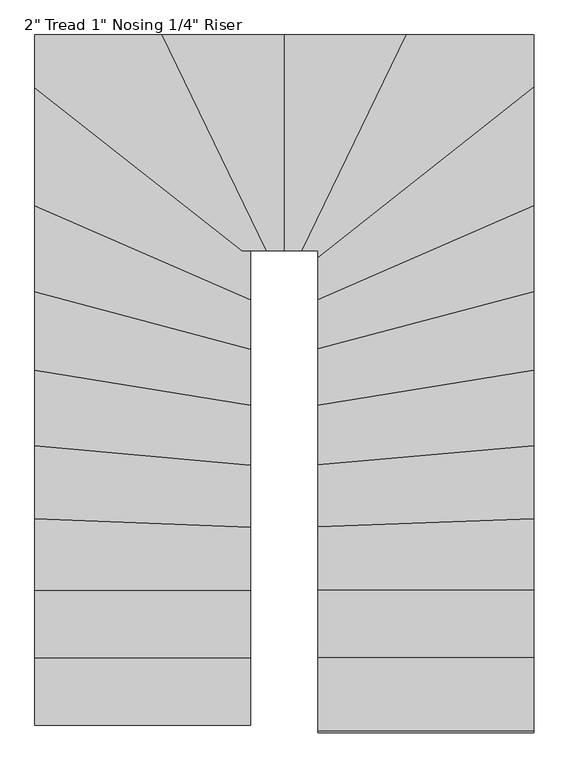
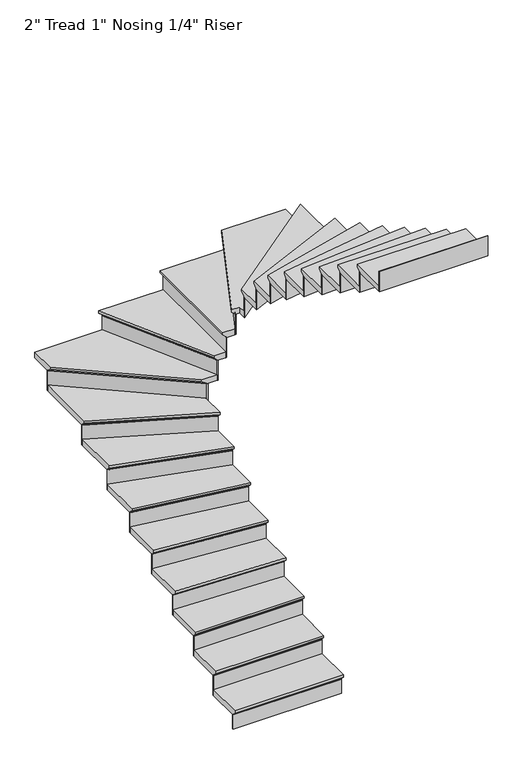
"""IFC4 building model written with IfcOpenShell, lengths in millimetres: stair flight geometry."""

from ifc_helpers import new_model, si_unit, origin, place, context, project, spatial, faceted_brep, source, transform, mapped, element, save


def stair_flight_b3d82c80(model_context):
    return source(origin(), model_context, "Body", "Brep", [
        faceted_brep([(-5047.1987704, -4554.2130548, 55019.1214286), (-5047.1987704, -4554.2130548, 55038.1714286), (-5940.8822214, -4554.2130548, 55038.1714286), (-5940.8822214, -4554.2130548, 55019.1214286), (-5047.1987704, -4528.8130548, 54993.7214286), (-5940.8822214, -4528.8130548, 54993.7214286), (-5047.1987704, -4249.4130548, 55038.1714286), (-5940.8822214, -4249.4130548, 55038.1714286), (-5940.8822214, -4528.8130548, 54987.3714286), (-5940.8822214, -4249.4130548, 54987.3714286), (-5047.1987704, -4249.4130548, 54987.3714286), (-5047.1987704, -4528.8130548, 54987.3714286)], [[[0, 1, 2, 3]], [[4, 0, 3, 5]], [[2, 1, 6, 7]], [[8, 9, 10, 11]], [[2, 7, 9, 8, 5, 3]], [[8, 11, 4, 5]], [[6, 1, 0, 4, 11, 10]], [[7, 6, 10, 9]]]),
        faceted_brep([(-5047.1987704, -4528.8130548, 54987.3714286), (-5047.1987704, -4528.8130548, 54864.0), (-5047.1987704, -4522.4630548, 54864.0), (-5047.1987704, -4522.4630548, 54987.3714286), (-5940.8822214, -4528.8130548, 54987.3714286), (-5940.8822214, -4522.4630548, 54987.3714286), (-5940.8822214, -4522.4630548, 54864.0), (-5940.8822214, -4528.8130548, 54864.0)], [[[0, 1, 2, 3]], [[4, 5, 6, 7]], [[1, 0, 4, 7]], [[2, 1, 7, 6]], [[3, 2, 6, 5]], [[0, 3, 5, 4]]]),
        faceted_brep([(-5047.1987704, -4249.4130548, 55161.5428571), (-5047.1987704, -4249.4130548, 54987.3714286), (-5047.1987704, -4243.0630548, 54987.3714286), (-5047.1987704, -4243.0630548, 55161.5428571), (-5940.8822214, -4249.4130548, 55161.5428571), (-5940.8822214, -4243.0630548, 55161.5428571), (-5940.8822214, -4243.0630548, 54987.3714286), (-5940.8822214, -4249.4130548, 54987.3714286)], [[[0, 1, 2, 3]], [[4, 5, 6, 7]], [[1, 0, 4, 7]], [[2, 1, 7, 6]], [[3, 2, 6, 5]], [[0, 3, 5, 4]]]),
        faceted_brep([(-5940.8822214, -4274.8130548, 55212.3428571), (-5047.1987704, -4274.8130548, 55212.3428571), (-5047.1987704, -3970.0130548, 55212.3428571), (-5940.8822214, -3970.0130548, 55212.3428571), (-5940.8822214, -4249.4130548, 55161.5428571), (-5940.8822214, -3970.0130548, 55161.5428571), (-5047.1987704, -3970.0130548, 55161.5428571), (-5047.1987704, -4249.4130548, 55161.5428571), (-5940.8822214, -4249.4130548, 55167.8928571), (-5940.8822214, -4274.8130548, 55193.2928571), (-5047.1987704, -4249.4130548, 55167.8928571), (-5047.1987704, -4274.8130548, 55193.2928571)], [[[0, 1, 2, 3]], [[4, 5, 6, 7]], [[0, 3, 5, 4, 8, 9]], [[4, 7, 10, 8]], [[2, 1, 11, 10, 7, 6]], [[3, 2, 6, 5]], [[11, 1, 0, 9]], [[10, 11, 9, 8]]]),
        faceted_brep([(-5047.1987704, -3970.0130548, 55335.7142857), (-5047.1987704, -3970.0130548, 55161.5428571), (-5047.1987704, -3963.6630548, 55161.5428571), (-5047.1987704, -3963.6630548, 55335.7142857), (-5940.8822214, -3970.0130548, 55335.7142857), (-5940.8822214, -3963.6630548, 55335.7142857), (-5940.8822214, -3963.6630548, 55161.5428571), (-5940.8822214, -3970.0130548, 55161.5428571)], [[[0, 1, 2, 3]], [[4, 5, 6, 7]], [[1, 0, 4, 7]], [[2, 1, 7, 6]], [[3, 2, 6, 5]], [[0, 3, 5, 4]]]),
        faceted_brep([(-5940.8822214, -3995.4130548, 55386.5142857), (-5047.1987704, -3995.4130548, 55386.5142857), (-5047.1987704, -3707.9036879, 55386.5142857), (-5940.8822214, -3673.2843203, 55386.5142857), (-5940.8822214, -3970.0130548, 55335.7142857), (-5940.8822214, -3673.2843203, 55335.7142857), (-5047.1987704, -3707.9036879, 55335.7142857), (-5047.1987704, -3970.0130548, 55335.7142857), (-5940.8822214, -3970.0130548, 55342.0642857), (-5940.8822214, -3995.4130548, 55367.4642857), (-5047.1987704, -3970.0130548, 55342.0642857), (-5047.1987704, -3995.4130548, 55367.4642857)], [[[0, 1, 2, 3]], [[4, 5, 6, 7]], [[0, 3, 5, 4, 8, 9]], [[4, 7, 10, 8]], [[2, 1, 11, 10, 7, 6]], [[3, 2, 6, 5]], [[11, 1, 0, 9]], [[10, 11, 9, 8]]]),
        faceted_brep([(-5047.1987704, -3707.9036879, 55509.8857143), (-5047.1987704, -3707.9036879, 55335.7142857), (-5047.1987704, -3701.5489252, 55335.7142857), (-5047.1987704, -3701.5489252, 55509.8857143), (-5940.8822214, -3673.2843203, 55509.8857143), (-5940.8822214, -3666.9295576, 55509.8857143), (-5940.8822214, -3666.9295576, 55335.7142857), (-5940.8822214, -3673.2843203, 55335.7142857)], [[[0, 1, 2, 3]], [[4, 5, 6, 7]], [[1, 0, 4, 7]], [[2, 1, 7, 6]], [[3, 2, 6, 5]], [[0, 3, 5, 4]]]),
        faceted_brep([(-5940.8822214, -3698.703371, 55560.6857143), (-5047.1987704, -3733.3227386, 55560.6857143), (-5047.1987704, -3451.3234819, 55560.6857143), (-5940.8822214, -3370.89733, 55560.6857143), (-5940.8822214, -3673.2843203, 55509.8857143), (-5940.8822214, -3370.89733, 55509.8857143), (-5047.1987704, -3451.3234819, 55509.8857143), (-5047.1987704, -3707.9036879, 55509.8857143), (-5940.8822214, -3673.2843203, 55516.2357143), (-5940.8822214, -3698.703371, 55541.6357143), (-5047.1987704, -3707.9036879, 55516.2357143), (-5047.1987704, -3733.3227386, 55541.6357143)], [[[0, 1, 2, 3]], [[4, 5, 6, 7]], [[0, 3, 5, 4, 8, 9]], [[4, 7, 10, 8]], [[2, 1, 11, 10, 7, 6]], [[3, 2, 6, 5]], [[11, 1, 0, 9]], [[10, 11, 9, 8]]]),
        faceted_brep([(-5047.1987704, -3451.3234819, 55684.0571429), (-5047.1987704, -3451.3234819, 55509.8857143), (-5047.1987704, -3444.9478197, 55509.8857143), (-5047.1987704, -3444.9478197, 55684.0571429), (-5940.8822214, -3370.89733, 55684.0571429), (-5940.8822214, -3364.5216678, 55684.0571429), (-5940.8822214, -3364.5216678, 55509.8857143), (-5940.8822214, -3370.89733, 55509.8857143)], [[[0, 1, 2, 3]], [[4, 5, 6, 7]], [[1, 0, 4, 7]], [[2, 1, 7, 6]], [[3, 2, 6, 5]], [[0, 3, 5, 4]]]),
        faceted_brep([(-5940.8822214, -3396.3999789, 55734.8571429), (-5047.1987704, -3476.8261308, 55734.8571429), (-5047.1987704, -3203.4301079, 55734.8571429), (-5940.8822214, -3059.5417727, 55734.8571429), (-5940.8822214, -3370.89733, 55684.0571429), (-5940.8822214, -3059.5417727, 55684.0571429), (-5047.1987704, -3203.4301079, 55684.0571429), (-5047.1987704, -3451.3234819, 55684.0571429), (-5940.8822214, -3370.89733, 55690.4071429), (-5940.8822214, -3396.3999789, 55715.8071429), (-5047.1987704, -3451.3234819, 55690.4071429), (-5047.1987704, -3476.8261308, 55715.8071429)], [[[0, 1, 2, 3]], [[4, 5, 6, 7]], [[0, 3, 5, 4, 8, 9]], [[4, 7, 10, 8]], [[2, 1, 11, 10, 7, 6]], [[3, 2, 6, 5]], [[11, 1, 0, 9]], [[10, 11, 9, 8]]]),
        faceted_brep([(-5047.1987704, -3203.4301079, 55858.2285714), (-5047.1987704, -3203.4301079, 55684.0571429), (-5047.1987704, -3196.9983292, 55684.0571429), (-5047.1987704, -3196.9983292, 55858.2285714), (-5940.8822214, -3059.5417727, 55858.2285714), (-5940.8822214, -3053.109994, 55858.2285714), (-5940.8822214, -3053.109994, 55684.0571429), (-5940.8822214, -3059.5417727, 55684.0571429)], [[[0, 1, 2, 3]], [[4, 5, 6, 7]], [[1, 0, 4, 7]], [[2, 1, 7, 6]], [[3, 2, 6, 5]], [[0, 3, 5, 4]]]),
        faceted_brep([(-5940.8822214, -3085.2688872, 55909.0285714), (-5047.1987704, -3229.1572224, 55909.0285714), (-5047.1987704, -2970.3553609, 55909.0285714), (-5940.8822214, -2732.7052783, 55909.0285714), (-5940.8822214, -3059.5417727, 55858.2285714), (-5940.8822214, -2732.7052783, 55858.2285714), (-5047.1987704, -2970.3553609, 55858.2285714), (-5047.1987704, -3203.4301079, 55858.2285714), (-5940.8822214, -3059.5417727, 55864.5785714), (-5940.8822214, -3085.2688872, 55889.9785714), (-5047.1987704, -3203.4301079, 55864.5785714), (-5047.1987704, -3229.1572224, 55889.9785714)], [[[0, 1, 2, 3]], [[4, 5, 6, 7]], [[0, 3, 5, 4, 8, 9]], [[4, 7, 10, 8]], [[2, 1, 11, 10, 7, 6]], [[3, 2, 6, 5]], [[11, 1, 0, 9]], [[10, 11, 9, 8]]]),
        faceted_brep([(-5047.1987704, -2970.3553609, 56032.4), (-5047.1987704, -2970.3553609, 55858.2285714), (-5047.1987704, -2963.7846771, 55858.2285714), (-5047.1987704, -2963.7846771, 56032.4), (-5940.8822214, -2732.7052783, 56032.4), (-5940.8822214, -2726.1345945, 56032.4), (-5940.8822214, -2726.1345945, 55858.2285714), (-5940.8822214, -2732.7052783, 55858.2285714)], [[[0, 1, 2, 3]], [[4, 5, 6, 7]], [[1, 0, 4, 7]], [[2, 1, 7, 6]], [[3, 2, 6, 5]], [[0, 3, 5, 4]]]),
        faceted_brep([(-5940.8822214, -2758.9880136, 56083.2), (-5047.1987704, -2996.6380961, 56083.2), (-5047.1987704, -2765.8050203, 56083.2), (-5940.8822214, -2375.5896532, 56083.2), (-5940.8822214, -2732.7052783, 56032.4), (-5940.8822214, -2375.5896532, 56032.4), (-5047.1987704, -2765.8050203, 56032.4), (-5047.1987704, -2970.3553609, 56032.4), (-5940.8822214, -2732.7052783, 56038.75), (-5940.8822214, -2758.9880136, 56064.15), (-5047.1987704, -2970.3553609, 56038.75), (-5047.1987704, -2996.6380961, 56064.15)], [[[0, 1, 2, 3]], [[4, 5, 6, 7]], [[0, 3, 5, 4, 8, 9]], [[4, 7, 10, 8]], [[2, 1, 11, 10, 7, 6]], [[3, 2, 6, 5]], [[11, 1, 0, 9]], [[10, 11, 9, 8]]]),
        faceted_brep([(-5047.1987704, -2765.8050203, 56206.5714286), (-5047.1987704, -2765.8050203, 56032.4), (-5047.1987704, -2758.8760908, 56032.4), (-5047.1987704, -2758.8760908, 56206.5714286), (-5940.8822214, -2375.5896532, 56206.5714286), (-5940.8822214, -2368.6607237, 56206.5714286), (-5940.8822214, -2368.6607237, 56032.4), (-5940.8822214, -2375.5896532, 56032.4)], [[[0, 1, 2, 3]], [[4, 5, 6, 7]], [[1, 0, 4, 7]], [[2, 1, 7, 6]], [[3, 2, 6, 5]], [[0, 3, 5, 4]]]),
        faceted_brep([(-5940.8822214, -2403.3053713, 56257.3714286), (-5047.1987704, -2793.5207384, 56257.3714286), (-5047.1987704, -2590.8424524, 56257.3714286), (-5040.8038639, -2590.8424524, 56257.3714286), (-5940.8822214, -1882.1944717, 56257.3714286), (-5940.8822214, -2375.5896532, 56206.5714286), (-5940.8822214, -1882.1944717, 56206.5714286), (-5040.8038639, -2590.8424524, 56206.5714286), (-5047.1987704, -2590.8424524, 56206.5714286), (-5047.1987704, -2765.8050203, 56206.5714286), (-5940.8822214, -2375.5896532, 56212.9214286), (-5940.8822214, -2403.3053713, 56238.3214286), (-5047.1987704, -2765.8050203, 56212.9214286), (-5047.1987704, -2793.5207384, 56238.3214286)], [[[0, 1, 2, 3, 4]], [[5, 6, 7, 8, 9]], [[0, 4, 6, 5, 10, 11]], [[5, 9, 12, 10]], [[2, 1, 13, 12, 9, 8]], [[4, 3, 7, 6]], [[13, 1, 0, 11]], [[12, 13, 11, 10]], [[3, 2, 8, 7]]]),
        faceted_brep([(-5040.8038639, -2590.8424524, 56380.7428571), (-5040.8038639, -2590.8424524, 56206.5714286), (-5030.5387554, -2590.8424524, 56206.5714286), (-5030.5387554, -2590.8424524, 56380.7428571), (-5940.8822214, -1882.1944717, 56380.7428571), (-5940.8822214, -1874.1125661, 56380.7428571), (-5940.8822214, -1874.1125661, 56206.5714286), (-5940.8822214, -1882.1944717, 56206.5714286)], [[[0, 1, 2, 3]], [[4, 5, 6, 7]], [[1, 0, 4, 7]], [[2, 1, 7, 6]], [[3, 2, 6, 5]], [[0, 3, 5, 4]]]),
        faceted_brep([(-5384.6489457, -1697.1590014, 56431.5428571), (-5940.8822214, -1697.1590014, 56431.5428571), (-5940.8822214, -1914.5220945, 56431.5428571), (-5081.8642978, -2590.8424524, 56431.5428571), (-4952.3566185, -2590.8424524, 56431.5428571), (-5940.8822214, -1697.1590014, 56380.7428571), (-5384.6489457, -1697.1590014, 56380.7428571), (-4952.3566185, -2590.8424524, 56380.7428571), (-5040.8038639, -2590.8424524, 56380.7428571), (-5940.8822214, -1882.1944717, 56380.7428571), (-5940.8822214, -1882.1944717, 56387.0928571), (-5940.8822214, -1914.5220945, 56412.4928571), (-5040.8038639, -2590.8424524, 56387.0928571), (-5081.8642978, -2590.8424524, 56412.4928571)], [[[0, 1, 2, 3, 4]], [[5, 6, 7, 8, 9]], [[1, 0, 6, 5]], [[2, 1, 5, 9, 10, 11]], [[9, 8, 12, 10]], [[4, 3, 13, 12, 8, 7]], [[0, 4, 7, 6]], [[13, 3, 2, 11]], [[12, 13, 11, 10]]]),
        faceted_brep([(-4952.3566185, -2590.8424524, 56554.9142857), (-4952.3566185, -2590.8424524, 56380.7428571), (-4945.3027294, -2590.8424524, 56380.7428571), (-4945.3027294, -2590.8424524, 56554.9142857), (-5384.6489457, -1697.1590014, 56554.9142857), (-5377.5950566, -1697.1590014, 56554.9142857), (-5377.5950566, -1697.1590014, 56380.7428571), (-5384.6489457, -1697.1590014, 56380.7428571)], [[[0, 1, 2, 3]], [[4, 5, 6, 7]], [[1, 0, 4, 7]], [[2, 1, 7, 6]], [[3, 2, 6, 5]], [[0, 3, 5, 4]]]),
        faceted_brep([(-5412.8645022, -1697.1590014, 56605.7142857), (-4980.5721749, -2590.8424524, 56605.7142857), (-4882.0987704, -2590.8424524, 56605.7142857), (-4882.0987706, -1697.1590014, 56605.7142857), (-5384.6489457, -1697.1590014, 56554.9142857), (-4882.0987706, -1697.1590014, 56554.9142857), (-4882.0987704, -2590.8424524, 56554.9142857), (-4952.3566185, -2590.8424524, 56554.9142857), (-5384.6489457, -1697.1590014, 56561.2642857), (-5412.8645022, -1697.1590014, 56586.6642857), (-4952.3566185, -2590.8424524, 56561.2642857), (-4980.5721749, -2590.8424524, 56586.6642857)], [[[0, 1, 2, 3]], [[4, 5, 6, 7]], [[0, 3, 5, 4, 8, 9]], [[4, 7, 10, 8]], [[3, 2, 6, 5]], [[11, 1, 0, 9]], [[10, 11, 9, 8]], [[2, 1, 11, 10, 7, 6]]]),
        faceted_brep([(-4882.0987704, -2590.8424524, 56729.0857143), (-4882.0987704, -2590.8424524, 56554.9142857), (-4875.7487704, -2590.8424524, 56554.9142857), (-4875.7487704, -2590.8424524, 56729.0857143), (-4882.0987706, -1697.1590014, 56729.0857143), (-4875.7487706, -1697.1590014, 56729.0857143), (-4875.7487706, -1697.1590014, 56554.9142857), (-4882.0987706, -1697.1590014, 56554.9142857)], [[[0, 1, 2, 3]], [[4, 5, 6, 7]], [[1, 0, 4, 7]], [[2, 1, 7, 6]], [[3, 2, 6, 5]], [[0, 3, 5, 4]]]),
        faceted_brep([(-4907.4987706, -1697.1590014, 56779.8857143), (-4907.4987704, -2590.8424524, 56779.8857143), (-4806.2098095, -2590.8424524, 56779.8857143), (-4373.9174828, -1697.1590014, 56779.8857143), (-4882.0987706, -1697.1590014, 56729.0857143), (-4373.9174828, -1697.1590014, 56729.0857143), (-4806.2098095, -2590.8424524, 56729.0857143), (-4882.0987704, -2590.8424524, 56729.0857143), (-4882.0987706, -1697.1590014, 56735.4357143), (-4907.4987706, -1697.1590014, 56760.8357143), (-4882.0987704, -2590.8424524, 56735.4357143), (-4907.4987704, -2590.8424524, 56760.8357143)], [[[0, 1, 2, 3]], [[4, 5, 6, 7]], [[0, 3, 5, 4, 8, 9]], [[4, 7, 10, 8]], [[2, 1, 11, 10, 7, 6]], [[3, 2, 6, 5]], [[11, 1, 0, 9]], [[10, 11, 9, 8]]]),
        faceted_brep([(-4806.2098095, -2590.8424524, 56903.2571429), (-4806.2098095, -2590.8424524, 56729.0857143), (-4799.1559204, -2590.8424524, 56729.0857143), (-4799.1559204, -2590.8424524, 56903.2571429), (-4373.9174828, -1697.1590014, 56903.2571429), (-4366.8635937, -1697.1590014, 56903.2571429), (-4366.8635937, -1697.1590014, 56729.0857143), (-4373.9174828, -1697.1590014, 56729.0857143)], [[[0, 1, 2, 3]], [[4, 5, 6, 7]], [[1, 0, 4, 7]], [[2, 1, 7, 6]], [[3, 2, 6, 5]], [[0, 3, 5, 4]]]),
        faceted_brep([(-3874.1153195, -1946.8497166, 56954.0571429), (-3874.1153195, -1697.1590014, 56954.0571429), (-4402.1330392, -1697.1590014, 56954.0571429), (-4834.4253659, -2590.8424524, 56954.0571429), (-4767.7987704, -2590.8424524, 56954.0571429), (-4767.7987704, -2650.4628721, 56954.0571429), (-3874.1153195, -1697.1590014, 56903.2571429), (-3874.1153195, -1946.8497166, 56903.2571429), (-4767.7987704, -2650.4628721, 56903.2571429), (-4767.7987704, -2590.8424524, 56903.2571429), (-4806.2098095, -2590.8424524, 56903.2571429), (-4373.9174828, -1697.1590014, 56903.2571429), (-4806.2098095, -2590.8424524, 56909.6071429), (-4373.9174828, -1697.1590014, 56909.6071429), (-4834.4253659, -2590.8424524, 56935.0071429), (-4402.1330392, -1697.1590014, 56935.0071429)], [[[0, 1, 2, 3, 4, 5]], [[6, 7, 8, 9, 10, 11]], [[1, 0, 7, 6]], [[11, 10, 12, 13]], [[4, 3, 14, 12, 10, 9]], [[5, 4, 9, 8]], [[0, 5, 8, 7]], [[14, 3, 2, 15]], [[12, 14, 15, 13]], [[2, 1, 6, 11, 13, 15]]]),
        faceted_brep([(-4767.7987704, -2650.4628721, 57077.4285714), (-4767.7987704, -2650.4628721, 56903.2571429), (-4767.7987704, -2658.5447778, 56903.2571429), (-4767.7987704, -2658.5447778, 57077.4285714), (-3874.1153195, -1946.8497166, 57077.4285714), (-3874.1153195, -1954.9316222, 57077.4285714), (-3874.1153195, -1954.9316222, 56903.2571429), (-3874.1153195, -1946.8497166, 56903.2571429)], [[[0, 1, 2, 3]], [[4, 5, 6, 7]], [[1, 0, 4, 7]], [[2, 1, 7, 6]], [[3, 2, 6, 5]], [[0, 3, 5, 4]]]),
        faceted_brep([(-3874.1153195, -1914.5220938, 57128.2285714), (-4767.7987704, -2618.1352494, 57128.2285714), (-4767.7987704, -2821.2364563, 57128.2285714), (-3874.1153195, -2431.0210889, 57128.2285714), (-3874.1153195, -1946.8497166, 57077.4285714), (-3874.1153195, -2431.0210889, 57077.4285714), (-4767.7987704, -2821.2364563, 57077.4285714), (-4767.7987704, -2650.4628721, 57077.4285714), (-3874.1153195, -1946.8497166, 57083.7785714), (-3874.1153195, -1914.5220938, 57109.1785714), (-4767.7987704, -2650.4628721, 57083.7785714), (-4767.7987704, -2618.1352494, 57109.1785714)], [[[0, 1, 2, 3]], [[4, 5, 6, 7]], [[0, 3, 5, 4, 8, 9]], [[4, 7, 10, 8]], [[2, 1, 11, 10, 7, 6]], [[3, 2, 6, 5]], [[11, 1, 0, 9]], [[10, 11, 9, 8]]]),
        faceted_brep([(-4767.7987704, -2821.2364563, 57251.6), (-4767.7987704, -2821.2364563, 57077.4285714), (-4767.7987704, -2828.1653858, 57077.4285714), (-4767.7987704, -2828.1653858, 57251.6), (-3874.1153195, -2431.0210889, 57251.6), (-3874.1153195, -2437.9500185, 57251.6), (-3874.1153195, -2437.9500185, 57077.4285714), (-3874.1153195, -2431.0210889, 57077.4285714)], [[[0, 1, 2, 3]], [[4, 5, 6, 7]], [[1, 0, 4, 7]], [[2, 1, 7, 6]], [[3, 2, 6, 5]], [[0, 3, 5, 4]]]),
        faceted_brep([(-3874.1153195, -2403.3053709, 57302.4), (-4767.7987704, -2793.5207382, 57302.4), (-4767.7987704, -3022.9208311, 57302.4), (-3874.1153195, -2785.2707484, 57302.4), (-3874.1153195, -2431.0210889, 57251.6), (-3874.1153195, -2785.2707484, 57251.6), (-4767.7987704, -3022.9208311, 57251.6), (-4767.7987704, -2821.2364563, 57251.6), (-3874.1153195, -2431.0210889, 57257.95), (-3874.1153195, -2403.3053709, 57283.35), (-4767.7987704, -2821.2364563, 57257.95), (-4767.7987704, -2793.5207382, 57283.35)], [[[0, 1, 2, 3]], [[4, 5, 6, 7]], [[0, 3, 5, 4, 8, 9]], [[4, 7, 10, 8]], [[2, 1, 11, 10, 7, 6]], [[3, 2, 6, 5]], [[11, 1, 0, 9]], [[10, 11, 9, 8]]]),
        faceted_brep([(-4767.7987704, -3022.9208311, 57425.7714286), (-4767.7987704, -3022.9208311, 57251.6), (-4767.7987704, -3029.4915149, 57251.6), (-4767.7987704, -3029.4915149, 57425.7714286), (-3874.1153195, -2785.2707484, 57425.7714286), (-3874.1153195, -2791.8414322, 57425.7714286), (-3874.1153195, -2791.8414322, 57251.6), (-3874.1153195, -2785.2707484, 57251.6)], [[[0, 1, 2, 3]], [[4, 5, 6, 7]], [[1, 0, 4, 7]], [[2, 1, 7, 6]], [[3, 2, 6, 5]], [[0, 3, 5, 4]]]),
        faceted_brep([(-3874.1153195, -2758.9880132, 57476.5714286), (-4767.7987704, -2996.6380959, 57476.5714286), (-4767.7987704, -3254.8843368, 57476.5714286), (-3874.1153195, -3110.9960015, 57476.5714286), (-3874.1153195, -2785.2707484, 57425.7714286), (-3874.1153195, -3110.9960015, 57425.7714286), (-4767.7987704, -3254.8843368, 57425.7714286), (-4767.7987704, -3022.9208311, 57425.7714286), (-3874.1153195, -2785.2707484, 57432.1214286), (-3874.1153195, -2758.9880132, 57457.5214286), (-4767.7987704, -3022.9208311, 57432.1214286), (-4767.7987704, -2996.6380959, 57457.5214286)], [[[0, 1, 2, 3]], [[4, 5, 6, 7]], [[0, 3, 5, 4, 8, 9]], [[4, 7, 10, 8]], [[2, 1, 11, 10, 7, 6]], [[3, 2, 6, 5]], [[11, 1, 0, 9]], [[10, 11, 9, 8]]]),
        faceted_brep([(-4767.7987704, -3254.8843368, 57599.9428571), (-4767.7987704, -3254.8843368, 57425.7714286), (-4767.7987704, -3261.3161154, 57425.7714286), (-4767.7987704, -3261.3161154, 57599.9428571), (-3874.1153195, -3110.9960015, 57599.9428571), (-3874.1153195, -3117.4277801, 57599.9428571), (-3874.1153195, -3117.4277801, 57425.7714286), (-3874.1153195, -3110.9960015, 57425.7714286)], [[[0, 1, 2, 3]], [[4, 5, 6, 7]], [[1, 0, 4, 7]], [[2, 1, 7, 6]], [[3, 2, 6, 5]], [[0, 3, 5, 4]]]),
        faceted_brep([(-3874.1153195, -3085.2688869, 57650.7428571), (-4767.7987704, -3229.1572222, 57650.7428571), (-4767.7987704, -3502.3287795, 57650.7428571), (-3874.1153195, -3421.9026274, 57650.7428571), (-3874.1153195, -3110.9960015, 57599.9428571), (-3874.1153195, -3421.9026274, 57599.9428571), (-4767.7987704, -3502.3287795, 57599.9428571), (-4767.7987704, -3254.8843368, 57599.9428571), (-3874.1153195, -3110.9960015, 57606.2928571), (-3874.1153195, -3085.2688869, 57631.6928571), (-4767.7987704, -3254.8843368, 57606.2928571), (-4767.7987704, -3229.1572222, 57631.6928571)], [[[0, 1, 2, 3]], [[4, 5, 6, 7]], [[0, 3, 5, 4, 8, 9]], [[4, 7, 10, 8]], [[2, 1, 11, 10, 7, 6]], [[3, 2, 6, 5]], [[11, 1, 0, 9]], [[10, 11, 9, 8]]]),
        faceted_brep([(-4767.7987704, -3502.3287795, 57774.1142857), (-4767.7987704, -3502.3287795, 57599.9428571), (-4767.7987704, -3508.7044417, 57599.9428571), (-4767.7987704, -3508.7044417, 57774.1142857), (-3874.1153195, -3421.9026274, 57774.1142857), (-3874.1153195, -3428.2782897, 57774.1142857), (-3874.1153195, -3428.2782897, 57599.9428571), (-3874.1153195, -3421.9026274, 57599.9428571)], [[[0, 1, 2, 3]], [[4, 5, 6, 7]], [[1, 0, 4, 7]], [[2, 1, 7, 6]], [[3, 2, 6, 5]], [[0, 3, 5, 4]]]),
        faceted_brep([(-3874.1153195, -3396.3999786, 57824.9142857), (-4767.7987704, -3476.8261306, 57824.9142857), (-4767.7987704, -3758.7417891, 57824.9142857), (-3874.1153195, -3724.1224215, 57824.9142857), (-3874.1153195, -3421.9026274, 57774.1142857), (-3874.1153195, -3724.1224215, 57774.1142857), (-4767.7987704, -3758.7417891, 57774.1142857), (-4767.7987704, -3502.3287795, 57774.1142857), (-3874.1153195, -3421.9026274, 57780.4642857), (-3874.1153195, -3396.3999786, 57805.8642857), (-4767.7987704, -3502.3287795, 57780.4642857), (-4767.7987704, -3476.8261306, 57805.8642857)], [[[0, 1, 2, 3]], [[4, 5, 6, 7]], [[0, 3, 5, 4, 8, 9]], [[4, 7, 10, 8]], [[2, 1, 11, 10, 7, 6]], [[3, 2, 6, 5]], [[11, 1, 0, 9]], [[10, 11, 9, 8]]]),
        faceted_brep([(-4767.7987704, -3758.7417891, 57948.2857143), (-4767.7987704, -3758.7417891, 57774.1142857), (-4767.7987704, -3765.0965518, 57774.1142857), (-4767.7987704, -3765.0965518, 57948.2857143), (-3874.1153195, -3724.1224215, 57948.2857143), (-3874.1153195, -3730.4771842, 57948.2857143), (-3874.1153195, -3730.4771842, 57774.1142857), (-3874.1153195, -3724.1224215, 57774.1142857)], [[[0, 1, 2, 3]], [[4, 5, 6, 7]], [[1, 0, 4, 7]], [[2, 1, 7, 6]], [[3, 2, 6, 5]], [[0, 3, 5, 4]]]),
        faceted_brep([(-3874.1153195, -3698.7033708, 57999.0857143), (-4767.7987704, -3733.3227384, 57999.0857143), (-4767.7987704, -4020.8130546, 57999.0857143), (-3874.1153195, -4020.8130546, 57999.0857143), (-3874.1153195, -3724.1224215, 57948.2857143), (-3874.1153195, -4020.8130546, 57948.2857143), (-4767.7987704, -4020.8130546, 57948.2857143), (-4767.7987704, -3758.7417891, 57948.2857143), (-3874.1153195, -3724.1224215, 57954.6357143), (-3874.1153195, -3698.7033708, 57980.0357143), (-4767.7987704, -3758.7417891, 57954.6357143), (-4767.7987704, -3733.3227384, 57980.0357143)], [[[0, 1, 2, 3]], [[4, 5, 6, 7]], [[0, 3, 5, 4, 8, 9]], [[4, 7, 10, 8]], [[2, 1, 11, 10, 7, 6]], [[3, 2, 6, 5]], [[11, 1, 0, 9]], [[10, 11, 9, 8]]]),
        faceted_brep([(-4767.7987704, -4020.8130546, 58122.4571429), (-4767.7987704, -4020.8130546, 57948.2857143), (-4767.7987704, -4027.1630546, 57948.2857143), (-4767.7987704, -4027.1630546, 58122.4571429), (-3874.1153195, -4020.8130546, 58122.4571429), (-3874.1153195, -4027.1630546, 58122.4571429), (-3874.1153195, -4027.1630546, 57948.2857143), (-3874.1153195, -4020.8130546, 57948.2857143)], [[[0, 1, 2, 3]], [[4, 5, 6, 7]], [[1, 0, 4, 7]], [[2, 1, 7, 6]], [[3, 2, 6, 5]], [[0, 3, 5, 4]]]),
        faceted_brep([(-3874.1153195, -3995.4130546, 58173.2571429), (-4767.7987704, -3995.4130546, 58173.2571429), (-4767.7987704, -4300.2130546, 58173.2571429), (-3874.1153195, -4300.2130546, 58173.2571429), (-3874.1153195, -4020.8130546, 58122.4571429), (-3874.1153195, -4300.2130546, 58122.4571429), (-4767.7987704, -4300.2130546, 58122.4571429), (-4767.7987704, -4020.8130546, 58122.4571429), (-3874.1153195, -4020.8130546, 58128.8071429), (-3874.1153195, -3995.4130546, 58154.2071429), (-4767.7987704, -4020.8130546, 58128.8071429), (-4767.7987704, -3995.4130546, 58154.2071429)], [[[0, 1, 2, 3]], [[4, 5, 6, 7]], [[0, 3, 5, 4, 8, 9]], [[4, 7, 10, 8]], [[2, 1, 11, 10, 7, 6]], [[3, 2, 6, 5]], [[11, 1, 0, 9]], [[10, 11, 9, 8]]]),
        faceted_brep([(-4767.7987704, -4300.2130546, 58296.6285714), (-4767.7987704, -4300.2130546, 58122.4571429), (-4767.7987704, -4306.5630546, 58122.4571429), (-4767.7987704, -4306.5630546, 58296.6285714), (-3874.1153195, -4300.2130546, 58296.6285714), (-3874.1153195, -4306.5630546, 58296.6285714), (-3874.1153195, -4306.5630546, 58122.4571429), (-3874.1153195, -4300.2130546, 58122.4571429)], [[[0, 1, 2, 3]], [[4, 5, 6, 7]], [[1, 0, 4, 7]], [[2, 1, 7, 6]], [[3, 2, 6, 5]], [[0, 3, 5, 4]]]),
        faceted_brep([(-4767.7987704, -4579.6130546, 58470.8), (-4767.7987704, -4579.6130546, 58296.6285714), (-4767.7987704, -4585.9630546, 58296.6285714), (-4767.7987704, -4585.9630546, 58470.8), (-3874.1153195, -4579.6130546, 58470.8), (-3874.1153195, -4585.9630546, 58470.8), (-3874.1153195, -4585.9630546, 58296.6285714), (-3874.1153195, -4579.6130546, 58296.6285714)], [[[0, 1, 2, 3]], [[4, 5, 6, 7]], [[1, 0, 4, 7]], [[2, 1, 7, 6]], [[3, 2, 6, 5]], [[0, 3, 5, 4]]]),
        faceted_brep([(-3874.1153195, -4274.8130546, 58347.4285714), (-4767.7987704, -4274.8130546, 58347.4285714), (-4767.7987704, -4579.6130546, 58347.4285714), (-3874.1153195, -4579.6130546, 58347.4285714), (-3874.1153195, -4300.2130546, 58296.6285714), (-3874.1153195, -4579.6130546, 58296.6285714), (-4767.7987704, -4579.6130546, 58296.6285714), (-4767.7987704, -4300.2130546, 58296.6285714), (-3874.1153195, -4300.2130546, 58302.9785714), (-3874.1153195, -4274.8130546, 58328.3785714), (-4767.7987704, -4300.2130546, 58302.9785714), (-4767.7987704, -4274.8130546, 58328.3785714)], [[[0, 1, 2, 3]], [[4, 5, 6, 7]], [[0, 3, 5, 4, 8, 9]], [[4, 7, 10, 8]], [[2, 1, 11, 10, 7, 6]], [[3, 2, 6, 5]], [[11, 1, 0, 9]], [[10, 11, 9, 8]]]),
    ])


if __name__ == "__main__":
    model = new_model("IFC4")
    model_context = context("Model", 3, world=origin())
    ifc_project = project(units=[si_unit("LENGTHUNIT", "METRE", prefix="MILLI")], contexts=[model_context])
    site = spatial("IfcSite", under=ifc_project)
    building = spatial("IfcBuilding", under=site)
    placement = place(None, origin())
    stair_flight_shape = stair_flight_b3d82c80(model_context)
    element("IfcStairFlight", 1, ObjectType="2\" Tread 1\" Nosing 1/4\" Riser", at=placement, inside=building, context=model_context, shape_type="MappedRepresentation", body=[
        mapped(stair_flight_shape, transform((0.0, 0.0, 0.0), x_axis=(1.0, 0.0, 0.0), y_axis=(0.0, 1.0, 0.0), z_axis=(0.0, 0.0, 1.0))),
    ])
    save(model, "model.ifc")

# Revit data of these elements
# Element 1 (IfcStairFlight, "2\" Tread 1\" Nosing 1/4\" Riser")
#   Materials on its faces: "Tile, Porcelain, 4in"
# Materials
#   "Tile, Porcelain, 4in": class "Generic", colour RGB 89 87 158, transparency 0, Description = "Porcelain tile, 4\", white", Cost = 0
